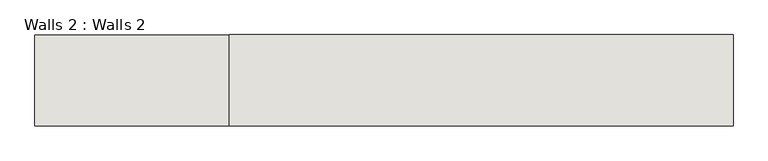
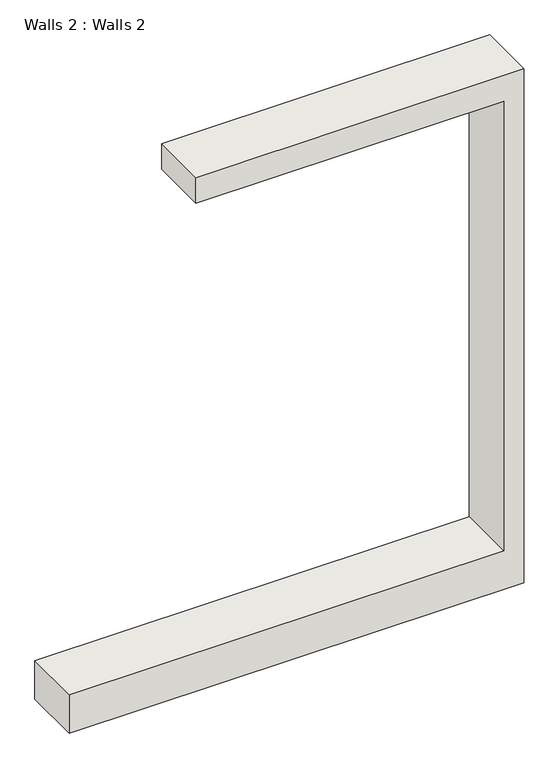
"""IFC4 building model written with IfcOpenShell, lengths in millimetres: wall geometry, Walls 2 : Walls 2."""

from ifc_helpers import new_model, si_unit, frame, origin, place, context, project, spatial, polyline, outline, extrude, source, transform, mapped, element, save


def walls_2_walls_2_e5515708(model_context):
    return source(origin(), model_context, "Body", "SweptSolid", [
        extrude(outline(polyline([(14630.4, -2546.1432037), (3962.4, -2546.1432037), (3962.4, -12299.7432037), (3048.0, -12299.7432037), (3048.0, -2088.9432037), (15240.0, -2088.9432037), (15240.0, -9454.9432037), (14630.4, -9454.9432037), (14630.4, -2546.1432037)])), frame((0.0, 40.8498736, 0.0), z_axis=(0.0, 1.0, 0.0), x_axis=(0.0, 0.0, 1.0)), (0.0, 0.0, 1.0), 1333.4050006),
    ])


if __name__ == "__main__":
    model = new_model("IFC4")
    model_context = context("Model", 3, world=origin())
    ifc_project = project(units=[si_unit("LENGTHUNIT", "METRE", prefix="MILLI")], contexts=[model_context])
    site = spatial("IfcSite", under=ifc_project)
    building = spatial("IfcBuilding", under=site)
    placement = place(None, origin())
    walls_2_walls_2_shape = walls_2_walls_2_e5515708(model_context)
    element("IfcWall", 1, ObjectType="Walls 2 : Walls 2", at=placement, inside=building, context=model_context, shape_type="MappedRepresentation", body=[
        mapped(walls_2_walls_2_shape, transform((0.0, 0.0, 0.0), x_axis=(1.0, 0.0, 0.0), y_axis=(0.0, 1.0, 0.0), z_axis=(0.0, 0.0, 1.0))),
    ])
    save(model, "model.ifc")

# Revit data of these elements
# Element 1 (IfcWall, "Walls 2 : Walls 2")
#   Materials on its faces: "Default Wall"
# Materials
#   "Default Wall": colour RGB 128 128 128, transparency 0
